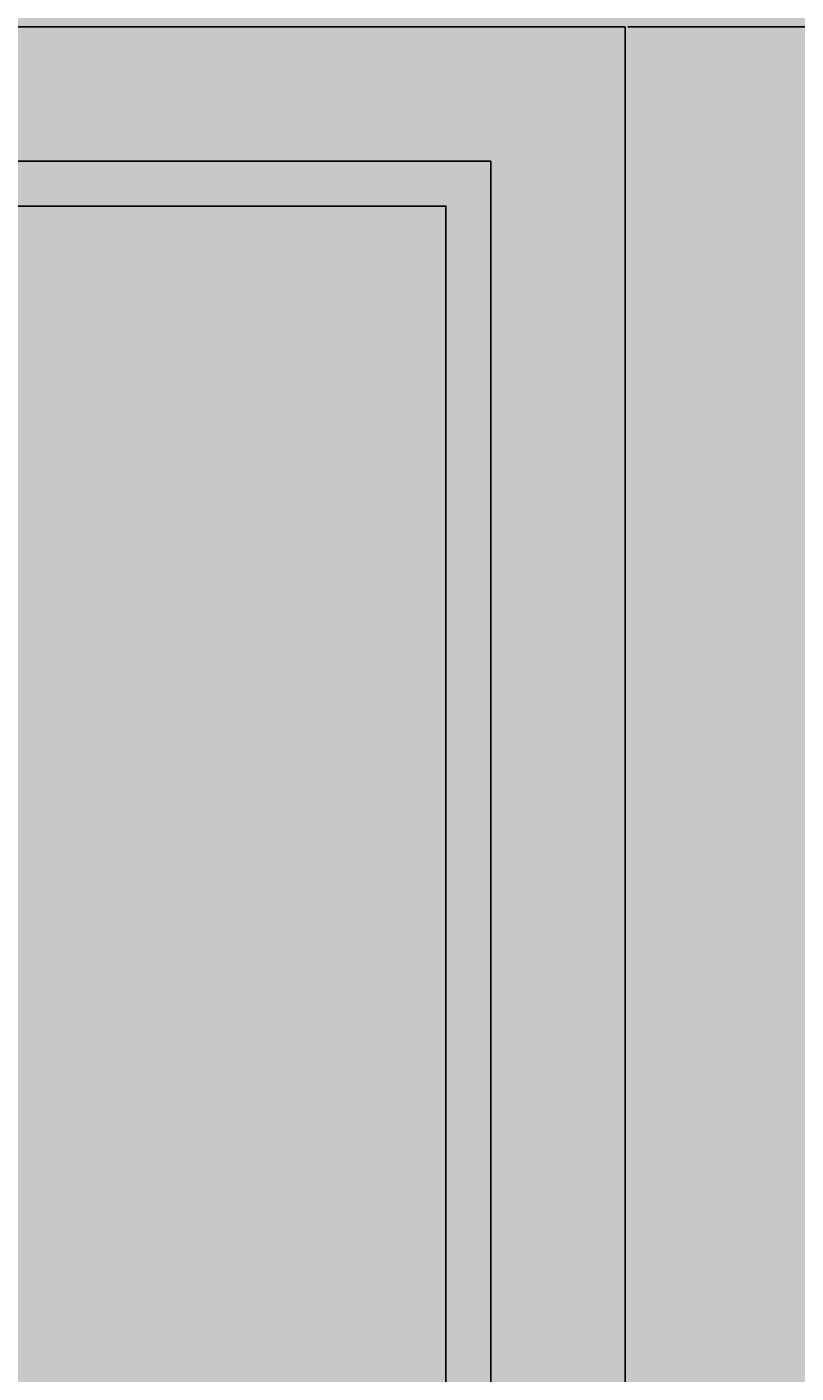
# Model space of a CAD drawing. Units: feet. Extents: x 2695 to 2912, y 795 to 1139.
# Tile 27 of 83: x 2825 to 2842, y 875 to 906. Entities that reach past the tile are written whole.
import ezdxf

# ---------------------------------------------------------------- set-up
doc = ezdxf.new("R2010")
doc.units = ezdxf.units.FT
for name, color, linetype, lineweight in [('A-ANNO-DIMS', 2, 'Continuous', 18), ('A-DOOR', 3, 'Continuous', 25), ('A-DOOR-PATT', 33, 'Continuous', 13), ('A-ELEV-PATT', 252, 'Continuous', 13)]:
    doc.layers.add(name, color=color, linetype=linetype, lineweight=lineweight)
doc.styles.get("Standard").update_dxf_attribs({"font": 'arial.ttf'})
doc.dimstyles.get("Standard").update_dxf_attribs({"dimtxt": 0.18, "dimasz": 0.18, "dimexe": 0.18, "dimexo": 0.0625, "dimgap": 0.09, "dimtad": 0, "dimtih": 1, "dimtoh": 1, "dimdec": 1, "dimzin": 0, "dimdsep": 46, "dimlunit": 3, "dimtxsty": 'Standard', "dimcen": 0.09, "dimadec": 0, "dimazin": 0, "dimtfac": 1, "dimtdec": 1, "dimtofl": 0, "dimtmove": 0, "dimatfit": 3, "dimfxl": 1, "dimtolj": 1, "dimtzin": 0, "dimarcsym": 0})

# ---------------------------------------------------------------- blocks, each defined once
blk = doc.blocks.new('*D14')
at = {"layer": 'A-ANNO-DIMS', "color": 0, "lineweight": -2, "transparency": 16777216}
for p, q in [((2838.439, 905.514), (2911.424, 905.514)), ((2911.244, 905.334), (2911.244, 890.368)), ((2911.244, 875.037), (2911.244, 890.004)), ((2758.214, 874.857), (2911.424, 874.857))]:
    blk.add_line(p, q, dxfattribs=at)
at = {"layer": 'A-ANNO-DIMS', "color": 0, "transparency": 16777216}
for points in [[(2911.214, 905.334), (2911.274, 905.334), (2911.244, 905.514)], [(2911.214, 875.037), (2911.274, 875.037), (2911.244, 874.857)]]:
    blk.add_solid(points, dxfattribs=at)
at = {"layer": 'Defpoints', "color": 0, "transparency": 16777216}
for p in [(2838.377, 905.514), (2911.244, 905.514), (2758.151, 874.857)]:
    blk.add_point(p, dxfattribs=at)
at = {"layer": 'A-ANNO-DIMS', "color": 0, "transparency": 16777216, "insert": (2911.244, 890.186), "char_height": 0.18, "attachment_point": 5}
blk.add_mtext('\\A1;30.66', dxfattribs=at)

msp = doc.modelspace()

# ---------------------------------------------------------------- hatches: boundary and pattern name
at = {"layer": 'A-DOOR-PATT'}
h = msp.add_hatch(color=256, dxfattribs=at)
h.set_gradient(color1=(211, 185, 150), color2=(211, 185, 150))
h.paths.add_polyline_path([(2805.9398, 905.5143), (2773.5029, 905.5143), (2773.5029, 810.9306), (2776.4999, 810.9306), (2776.4999, 902.5174), (2802.9429, 902.5174), (2802.9429, 810.9306), (2805.9398, 810.9306)])
h.paths.add_polyline_path([(2803.9681, 874.1057), (2805.0538, 874.1057), (2805.0538, 846.2857), (2803.9681, 846.2857)], flags=16)
h.paths.add_polyline_path([(2838.3767, 905.5143), (2805.9398, 905.5143), (2805.9398, 810.9306), (2808.9368, 810.9306), (2808.9368, 902.5174), (2835.3798, 902.5174), (2835.3798, 810.9306), (2838.3767, 810.9306)])
h = msp.add_hatch(color=256, dxfattribs=at)
h.set_gradient(color1=(211, 185, 150), color2=(211, 185, 150))
h.paths.add_polyline_path([(2777.5029, 901.5143), (2801.9398, 901.5143), (2801.9398, 810.9306), (2802.9429, 810.9306), (2802.9429, 902.5174), (2776.4999, 902.5174), (2776.4999, 810.9306), (2777.5029, 810.9306)])
h.paths.add_polyline_path([(2809.9398, 901.5143), (2834.3767, 901.5143), (2834.3767, 810.9306), (2835.3798, 810.9306), (2835.3798, 902.5174), (2808.9368, 902.5174), (2808.9368, 810.9306), (2809.9398, 810.9306)])
h = msp.add_hatch(color=256, dxfattribs=at)
h.set_gradient(color1=(173, 221, 247), color2=(173, 221, 247))
h.paths.add_polyline_path([(2801.9398, 901.5143), (2777.5029, 901.5143), (2777.5029, 810.9306), (2801.9398, 810.9306)])
h.paths.add_polyline_path([(2834.3767, 901.5143), (2809.9398, 901.5143), (2809.9398, 810.9306), (2834.3767, 810.9306)])
at = {"layer": 'A-ELEV-PATT'}
h = msp.add_hatch(color=256, dxfattribs=at)
h.set_gradient(color1=(147, 149, 152), color2=(147, 149, 152), tint=1)
h.paths.add_polyline_path([(2770.6361, 1118.4096), (2710.6361, 1118.4096), (2710.6361, 1062.9306), (2770.6361, 1062.9306)])
h.paths.add_polyline_path([(2890.6361, 1103.3378), (2770.6361, 1103.3378), (2770.6361, 1062.9306), (2890.6361, 1062.9306)])
h.paths.add_polyline_path([(2730.7081, 1048.1052), (2755.1125, 1048.1052), (2755.1125, 936.9306), (2770.6361, 936.9306), (2770.6361, 1050.3105), (2715.8852, 1050.3105), (2715.8852, 936.9306), (2730.7081, 936.9306)])
h.paths.add_polyline_path([(2890.6361, 1050.3105), (2770.6361, 1050.3105), (2770.6361, 971.9673), (2778.0341, 971.9673), (2778.0341, 1020.8235), (2843.575, 1020.8235), (2843.575, 971.9673), (2890.6361, 971.9673)])
h.paths.add_polyline_path([(2888.1882, 970.7156), (2843.575, 970.7156), (2843.575, 964.8267), (2888.1882, 964.8267)])
h.paths.add_polyline_path([(2888.1882, 964.1328), (2843.575, 964.1328), (2843.575, 956.614), (2888.1882, 956.614)])
h.paths.add_polyline_path([(2888.1882, 955.9202), (2843.575, 955.9202), (2843.575, 949.2892), (2888.1882, 949.2892)])
h.paths.add_polyline_path([(2888.1882, 948.5954), (2843.575, 948.5954), (2843.575, 941.3507), (2888.1882, 941.3507)])
h.paths.add_polyline_path([(2888.1882, 940.6569), (2843.575, 940.6569), (2843.575, 936.9306), (2888.1882, 936.9306)])
h.paths.add_polyline_path([(2890.6361, 970.7156), (2888.9368, 970.7156), (2888.9368, 964.8267), (2890.6361, 964.8267)])
h.paths.add_polyline_path([(2890.6361, 964.1328), (2888.9368, 964.1328), (2888.9368, 956.614), (2890.6361, 956.614)])
h.paths.add_polyline_path([(2890.6361, 955.9202), (2888.9368, 955.9202), (2888.9368, 949.2892), (2890.6361, 949.2892)])
h.paths.add_polyline_path([(2890.6361, 940.6569), (2888.9368, 940.6569), (2888.9368, 936.9306), (2890.6361, 936.9306)])
h.paths.add_polyline_path([(2890.6361, 948.5954), (2888.9368, 948.5954), (2888.9368, 941.3507), (2890.6361, 941.3507)])
h.paths.add_polyline_path([(2772.5216, 970.7156), (2770.6361, 970.7156), (2770.6361, 964.8267), (2772.5216, 964.8267)])
h.paths.add_polyline_path([(2772.5216, 964.1328), (2770.6361, 964.1328), (2770.6361, 956.614), (2772.5216, 956.614)])
h.paths.add_polyline_path([(2772.5216, 955.9202), (2770.6361, 955.9202), (2770.6361, 949.2892), (2772.5216, 949.2892)])
h.paths.add_polyline_path([(2772.5216, 948.5954), (2770.6361, 948.5954), (2770.6361, 941.3507), (2772.5216, 941.3507)])
h.paths.add_polyline_path([(2772.5216, 940.6569), (2770.6361, 940.6569), (2770.6361, 936.9306), (2772.5216, 936.9306)])
h.paths.add_polyline_path([(2778.0341, 940.6569), (2773.2702, 940.6569), (2773.2702, 936.9306), (2778.0341, 936.9306)])
h.paths.add_polyline_path([(2778.0341, 970.7156), (2773.2702, 970.7156), (2773.2702, 964.8267), (2778.0341, 964.8267)])
h.paths.add_polyline_path([(2778.0341, 964.1328), (2773.2702, 964.1328), (2773.2702, 956.614), (2778.0341, 956.614)])
h.paths.add_polyline_path([(2778.0341, 955.9202), (2773.2702, 955.9202), (2773.2702, 949.2892), (2778.0341, 949.2892)])
h.paths.add_polyline_path([(2778.0341, 948.5954), (2773.2702, 948.5954), (2773.2702, 941.3507), (2778.0341, 941.3507)])
h.paths.add_polyline_path([(2810.0407, 940.6569), (2780.0341, 940.6569), (2780.0341, 936.9306), (2810.0407, 936.9306)])
h.paths.add_polyline_path([(2890.6361, 924.3105), (2770.6361, 924.3105), (2770.6361, 810.9306), (2773.5029, 810.9306), (2773.5029, 905.5143), (2805.9398, 905.5143), (2838.3767, 905.5143), (2838.3767, 810.9306), (2890.6361, 810.9306)])

# ---------------------------------------------------------------- linework, layer by layer
at = {"layer": 'A-DOOR'}
for points in [[(2773.5029, 905.5143), (2838.3767, 905.5143), (2838.3767, 810.9306), (2773.5029, 810.9306)], [(2808.9368, 902.5174), (2835.3798, 902.5174), (2835.3798, 810.9306), (2808.9368, 810.9306)], [(2809.9398, 901.5143), (2834.3767, 901.5143), (2834.3767, 810.9306), (2809.9398, 810.9306)]]:
    msp.add_lwpolyline(points, close=True, dxfattribs=at)
for points in [[(2838.3767, 810.9306), (2838.3767, 905.5143), (2805.9398, 905.5143), (2805.9398, 810.9306)], [(2835.3798, 810.9306), (2835.3798, 902.5174), (2808.9368, 902.5174), (2808.9368, 810.9306)], [(2834.3767, 810.9306), (2834.3767, 901.5143), (2809.9398, 901.5143), (2809.9398, 810.9306)]]:
    msp.add_lwpolyline(points, dxfattribs=at)

# ---------------------------------------------------------------- dimensions: what is measured, and where the dimension line sits
at = {"layer": 'A-ANNO-DIMS'}
dim = msp.add_linear_dim(base=(2911.2444, 905.5143), p1=(2758.1515, 874.8571), p2=(2838.3767, 905.5143), angle=90, dimstyle='Standard', override={"dimdec": 2, "dimlfac": 1, "dimrnd": 0, "dimzin": 0, "dimdsep": 46, "dimlunit": 2}, dxfattribs=at)
dim.commit()
dim.dimension.update_dxf_attribs({"geometry": '*D14', "text_midpoint": (2911.2444, 890.1857)})

doc.saveas('drawing.dxf')
